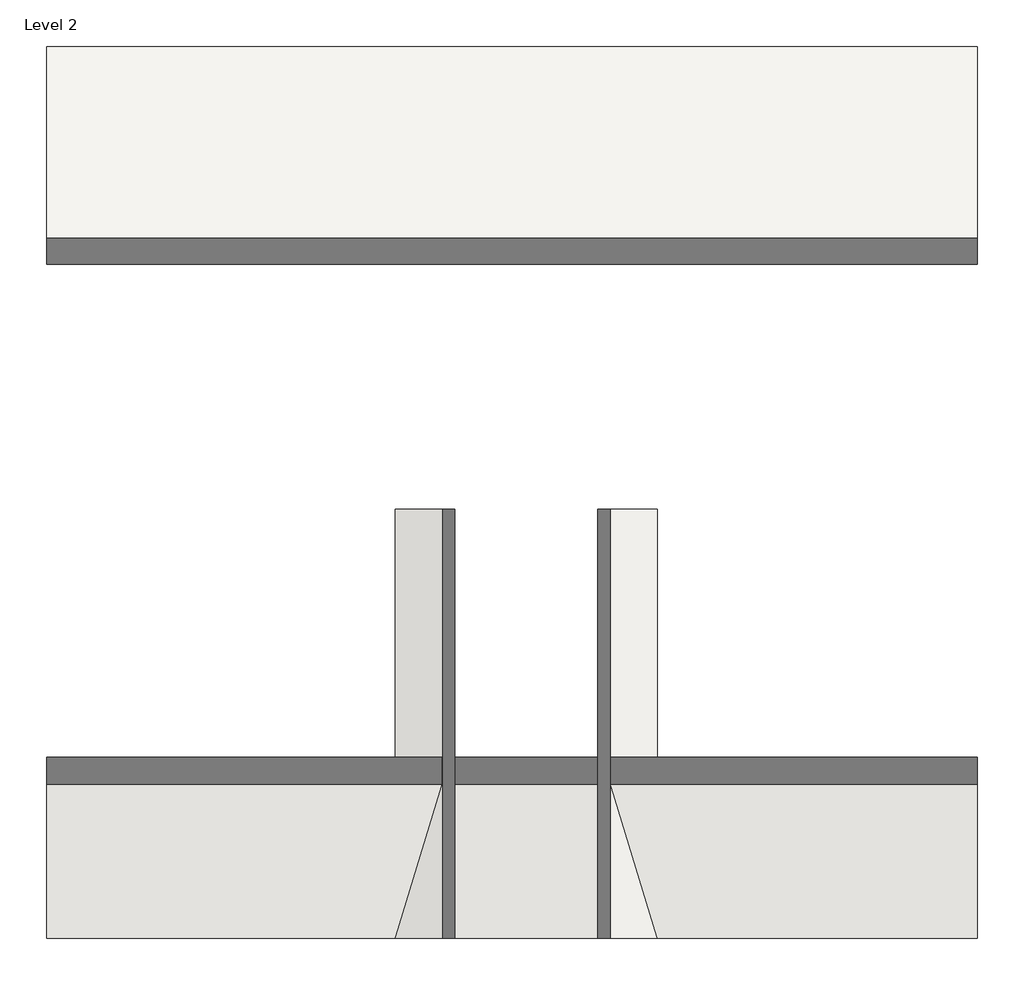
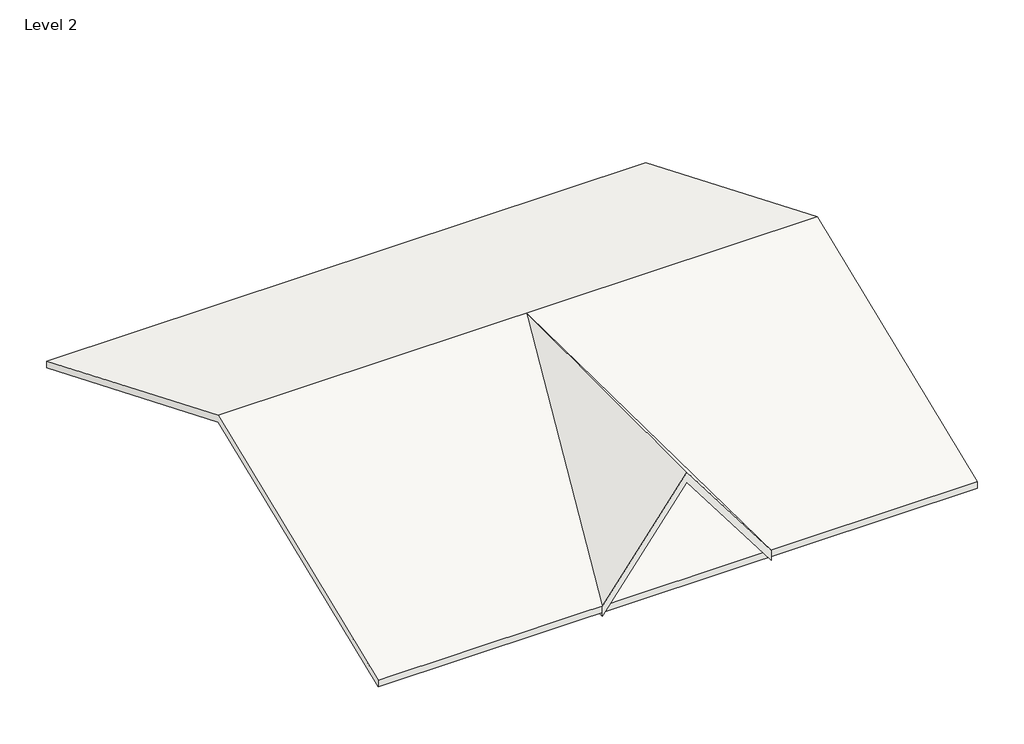
# One storey: 2 roofs.
"""IFC4 building model written with IfcOpenShell, lengths in millimetres."""

from ifc_helpers import new_model, si_unit, frame, origin, place, context, project, spatial, polyline, outline, extrude, element, save

model = new_model("IFC4")

# Units and contexts
model_context = context("Model", 3, world=origin())
ifc_project = project(units=[si_unit("LENGTHUNIT", "METRE", prefix="MILLI")], contexts=[model_context])

# Site, building, storey
site = spatial("IfcSite", under=ifc_project)
building = spatial("IfcBuilding", under=site)
storey = spatial("IfcBuildingStorey", under=building, Name="Level 2", Elevation=3048.0)

# Roofs
placement = place(None, origin())
element("IfcRoof", 1, ObjectType="6\"", at=placement, inside=storey, context=model_context, shape_type="SweptSolid", body=[
    extrude(outline(polyline([(2519.9899709, 3301.0664699), (9060.4899709, 5943.6), (16070.8899709, 3048.0), (16070.8899709, 2883.1115868), (9059.8538949, 5778.9743138), (2519.9899709, 3136.6977751), (2519.9899709, 3301.0664699)])), frame((-4714.3015363, 0.0, 0.0), z_axis=(1.0, 0.0, 0.0), x_axis=(0.0, 1.0, 0.0)), (0.0, 0.0, 1.0), 14144.625),
])
element("IfcRoof", 2, ObjectType="6\"", at=placement, inside=storey, context=model_context, shape_type="SweptSolid", body=[
    extrude(outline(polyline([(3301.0664699, 581.0316196), (3047.8325124, 581.0316196), (5690.3660425, 2572.3234637), (3047.8325124, 4563.6153078), (3301.0664699, 4563.6153078), (5943.6, 2572.3234637), (3301.0664699, 581.0316196)])), frame((0.0, 2519.9899709, 0.0), z_axis=(0.0, 1.0, 0.0), x_axis=(0.0, 0.0, 1.0)), (0.0, 0.0, 1.0), 6518.157413),
])

save(model, "model.ifc")

# Revit data of these elements
# Type "6\""
#   Assembly Code = "B1020"
#   Layers, outside or top first: 0' - 6" no material (function 1)
# Elements 1, 2 (IfcRoof, "6\"")
#   built-in parameter 1001710 = 33615
#   Phase Created = New Construction
#   Materials on its faces: "Default Roof"
# Materials
#   "Default Roof": colour RGB 88 101 114, transparency 0, Cost = 0
